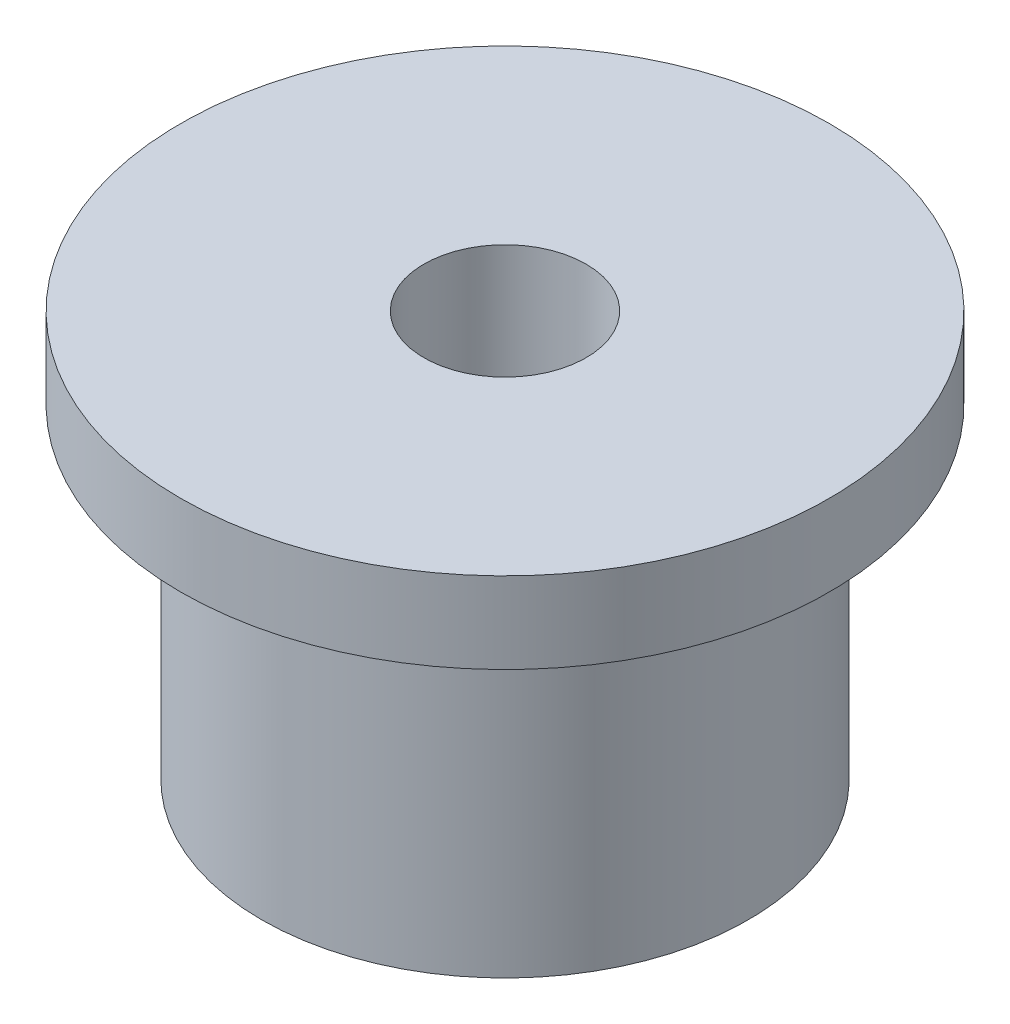
from build123d import *


with BuildPart() as part:
    # Bushing Half-Section Profile → Flanged Bushing Body (revolve)
    with BuildSketch(Plane(origin=(0, 0, 0), x_dir=(0, 0, -1), z_dir=(1, 0, 0))):
        Polygon((25, 0), (25, 125), (100, 125), (100, 100), (75, 100), (75, 0), align=None)
    revolve(axis=Axis((0, 0, 0), (0, 1, 0)))


solid = part.part
